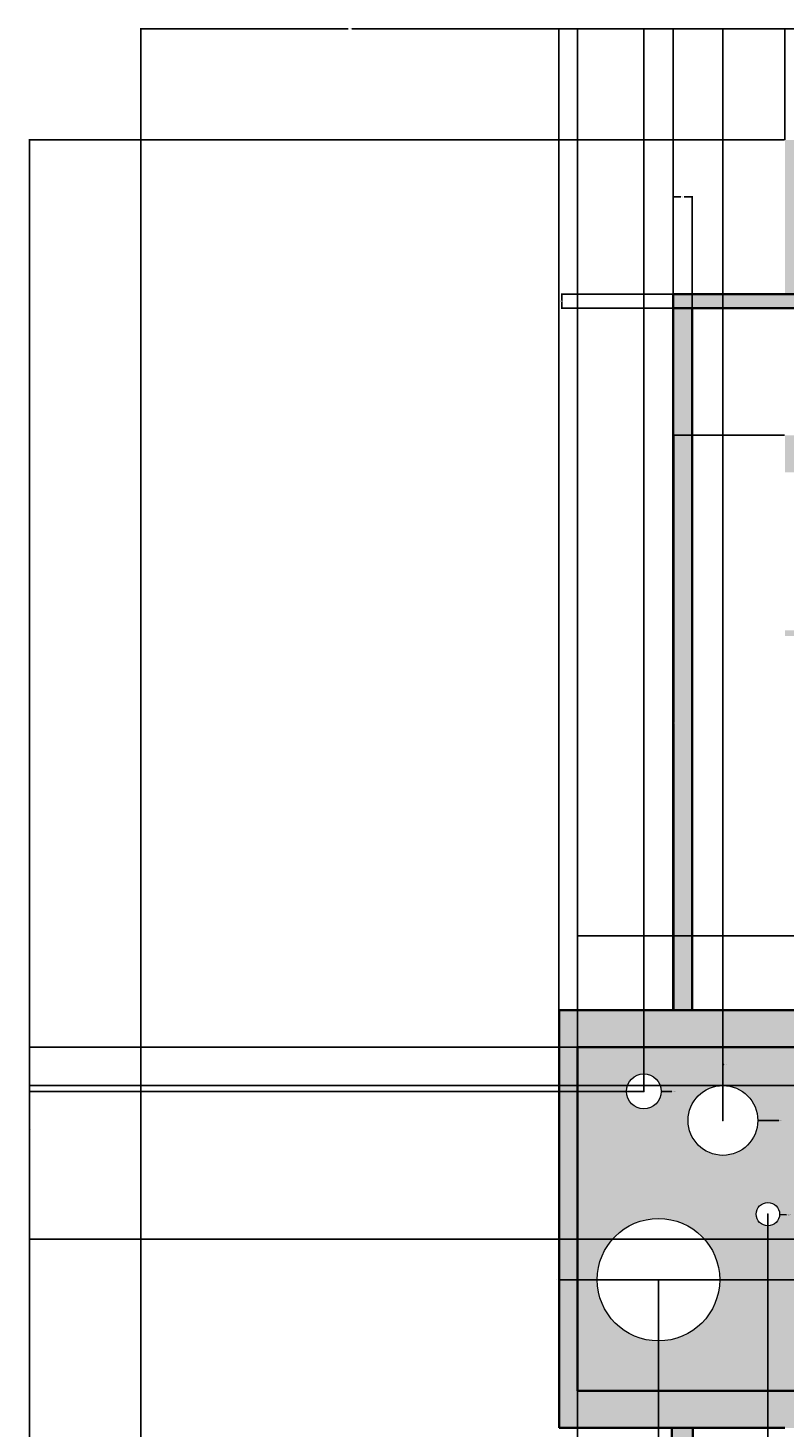
# Model space of a CAD drawing. Units: inches. Extents: x 73 to 607, y 92 to 651.
# Tile 13 of 18: x 73 to 256, y 311 to 651. Entities that reach past the tile are written whole.
import ezdxf

# ---------------------------------------------------------------- set-up
doc = ezdxf.new("R2010")
doc.units = ezdxf.units.IN
doc.header["$MEASUREMENT"] = 0
for name, color, linetype, lineweight in [('A-ANNO-DIMS', 2, 'Continuous', 18), ('A-ELEV', 7, 'Continuous', 35), ('A-ELEV-PANL', 7, 'Continuous', 18), ('A-ELEV-PATT-BKGD', 252, 'Continuous', 13), ('A-ELEV-PATT-SHAD', 8, 'Continuous', 13), ('A-ELEV-PATT-STON', 42, 'Continuous', 13), ('A-ELEV-PATT-WOOD', 32, 'Continuous', 13)]:
    doc.layers.add(name, color=color, linetype=linetype, lineweight=lineweight)
doc.styles.get("Standard").update_dxf_attribs({"font": 'arial.ttf'})
doc.dimstyles.get("Standard").update_dxf_attribs({"dimtxt": 0.18, "dimasz": 0.18, "dimexe": 0.18, "dimexo": 0.0625, "dimgap": 0.09, "dimtad": 0, "dimtih": 1, "dimtoh": 1, "dimdec": 4, "dimzin": 0, "dimdsep": 46, "dimtxsty": 'Standard', "dimcen": 0.09, "dimadec": 0, "dimazin": 0, "dimtfac": 1, "dimtdec": 4, "dimtofl": 0, "dimtmove": 0, "dimatfit": 3, "dimfxl": 1, "dimtolj": 1, "dimtzin": 0, "dimarcsym": 0})

# ---------------------------------------------------------------- blocks, each defined once
blk = doc.blocks.new('*D5')
at = {"layer": 'A-ANNO-DIMS', "color": 0, "lineweight": -2, "transparency": 16777216}
for p, q in [((256.41, 623.8), (72.92, 623.8)), ((73.1, 623.62), (73.1, 383.68)), ((73.1, 143.38), (73.1, 383.32)), ((100.04, 143.2), (72.92, 143.2))]:
    blk.add_line(p, q, dxfattribs=at)
at = {"layer": 'A-ANNO-DIMS', "color": 0, "transparency": 16777216}
for points in [[(73.07, 623.62), (73.13, 623.62), (73.1, 623.8)], [(73.07, 143.38), (73.13, 143.38), (73.1, 143.2)]]:
    blk.add_solid(points, dxfattribs=at)
at = {"layer": 'Defpoints', "color": 0, "transparency": 16777216}
for p in [(73.1, 623.8), (256.47, 623.8), (100.1, 143.2)]:
    blk.add_point(p, dxfattribs=at)
at = {"layer": 'A-ANNO-DIMS', "color": 0, "transparency": 16777216, "insert": (73.1, 383.5), "char_height": 0.18, "attachment_point": 5}
blk.add_mtext('\\A1;480.6', dxfattribs=at)
blk = doc.blocks.new('*D6')
at = {"layer": 'A-ANNO-DIMS', "color": 0, "lineweight": -2, "transparency": 16777216}
for p, q in [((100.1, 281.67), (100.1, 650.98)), ((100.28, 650.8), (150.41, 650.8)), ((201.45, 650.8), (151.32, 650.8)), ((201.63, 412.7), (201.63, 650.98))]:
    blk.add_line(p, q, dxfattribs=at)
at = {"layer": 'A-ANNO-DIMS', "color": 0, "transparency": 16777216}
for points in [[(100.28, 650.83), (100.28, 650.77), (100.1, 650.8)], [(201.45, 650.83), (201.45, 650.77), (201.63, 650.8)]]:
    blk.add_solid(points, dxfattribs=at)
at = {"layer": 'Defpoints', "color": 0, "transparency": 16777216}
for p in [(201.63, 650.8), (201.63, 412.64), (100.1, 281.6)]:
    blk.add_point(p, dxfattribs=at)
at = {"layer": 'A-ANNO-DIMS', "color": 0, "transparency": 16777216, "insert": (150.87, 650.8), "char_height": 0.18, "attachment_point": 5}
blk.add_mtext('\\A1;101.54', dxfattribs=at)
blk = doc.blocks.new('*D7')
at = {"layer": 'A-ANNO-DIMS', "color": 0, "lineweight": -2, "transparency": 16777216}
for p, q in [((201.63, 412.7), (201.63, 650.98)), ((201.81, 650.8), (215.01, 650.8)), ((229.14, 650.8), (215.94, 650.8)), ((229.32, 586.46), (229.32, 650.98))]:
    blk.add_line(p, q, dxfattribs=at)
at = {"layer": 'A-ANNO-DIMS', "color": 0, "transparency": 16777216}
for points in [[(201.81, 650.83), (201.81, 650.77), (201.63, 650.8)], [(229.14, 650.83), (229.14, 650.77), (229.32, 650.8)]]:
    blk.add_solid(points, dxfattribs=at)
at = {"layer": 'Defpoints', "color": 0, "transparency": 16777216}
for p in [(229.32, 650.8), (229.32, 586.39), (201.63, 412.64)]:
    blk.add_point(p, dxfattribs=at)
at = {"layer": 'A-ANNO-DIMS', "color": 0, "transparency": 16777216, "insert": (215.48, 650.8), "char_height": 0.18, "attachment_point": 5}
blk.add_mtext('\\A1;27.683', dxfattribs=at)
blk = doc.blocks.new('*D8')
at = {"layer": 'A-ANNO-DIMS', "color": 0, "lineweight": -2, "transparency": 16777216}
for p, q in [((229.32, 586.46), (229.32, 650.98)), ((229.5, 650.8), (242.43, 650.8)), ((256.29, 650.8), (243.36, 650.8)), ((256.47, 623.86), (256.47, 650.98))]:
    blk.add_line(p, q, dxfattribs=at)
at = {"layer": 'A-ANNO-DIMS', "color": 0, "transparency": 16777216}
for points in [[(229.5, 650.83), (229.5, 650.77), (229.32, 650.8)], [(256.29, 650.83), (256.29, 650.77), (256.47, 650.8)]]:
    blk.add_solid(points, dxfattribs=at)
at = {"layer": 'Defpoints', "color": 0, "transparency": 16777216}
for p in [(256.47, 650.8), (256.47, 623.8), (229.32, 586.39)]:
    blk.add_point(p, dxfattribs=at)
at = {"layer": 'A-ANNO-DIMS', "color": 0, "transparency": 16777216, "insert": (242.9, 650.8), "char_height": 0.18, "attachment_point": 5}
blk.add_mtext('\\A1;27.155', dxfattribs=at)
blk = doc.blocks.new('*D41')
at = {"layer": 'A-ANNO-DIMS', "color": 0, "lineweight": -2, "transparency": 16777216}
for p, q in [((229.26, 586.39), (202.14, 586.39)), ((202.32, 586.21), (202.32, 584.86)), ((202.32, 583.15), (202.32, 584.5)), ((229.26, 582.97), (202.14, 582.97))]:
    blk.add_line(p, q, dxfattribs=at)
at = {"layer": 'A-ANNO-DIMS', "color": 0, "transparency": 16777216}
for points in [[(202.29, 586.21), (202.35, 586.21), (202.32, 586.39)], [(202.29, 583.15), (202.35, 583.15), (202.32, 582.97)]]:
    blk.add_solid(points, dxfattribs=at)
at = {"layer": 'Defpoints', "color": 0, "transparency": 16777216}
for p in [(202.32, 586.39), (229.32, 586.39), (229.32, 582.97)]:
    blk.add_point(p, dxfattribs=at)
at = {"layer": 'A-ANNO-DIMS', "color": 0, "transparency": 16777216, "insert": (202.32, 584.68), "char_height": 0.18, "attachment_point": 5}
blk.add_mtext('\\A1;3.421', dxfattribs=at)
blk = doc.blocks.new('*D42')
at = {"layer": 'A-ANNO-DIMS', "color": 0, "lineweight": -2, "transparency": 16777216}
for p, q in [((229.32, 583.03), (229.32, 610.15)), ((229.5, 609.97), (231.22, 609.97)), ((233.74, 609.97), (232.02, 609.97)), ((233.92, 583.03), (233.92, 610.15))]:
    blk.add_line(p, q, dxfattribs=at)
at = {"layer": 'A-ANNO-DIMS', "color": 0, "transparency": 16777216}
for points in [[(229.5, 610), (229.5, 609.94), (229.32, 609.97)], [(233.74, 610), (233.74, 609.94), (233.92, 609.97)]]:
    blk.add_solid(points, dxfattribs=at)
at = {"layer": 'Defpoints', "color": 0, "transparency": 16777216}
for p in [(233.92, 609.97), (229.32, 582.97), (233.92, 582.97)]:
    blk.add_point(p, dxfattribs=at)
at = {"layer": 'A-ANNO-DIMS', "color": 0, "transparency": 16777216, "insert": (231.62, 609.97), "char_height": 0.18, "attachment_point": 5}
blk.add_mtext('\\A1;4.606', dxfattribs=at)
blk = doc.blocks.new('*D45')
at = {"layer": 'A-ANNO-DIMS', "color": 0, "lineweight": -2, "transparency": 16777216}
for p, q in [((256.41, 552.16), (229.29, 552.16)), ((229.47, 551.98), (229.47, 482.58)), ((229.47, 412.82), (229.47, 482.21)), ((256.41, 412.64), (229.29, 412.64))]:
    blk.add_line(p, q, dxfattribs=at)
at = {"layer": 'A-ANNO-DIMS', "color": 0, "transparency": 16777216}
for points in [[(229.44, 551.98), (229.5, 551.98), (229.47, 552.16)], [(229.44, 412.82), (229.5, 412.82), (229.47, 412.64)]]:
    blk.add_solid(points, dxfattribs=at)
at = {"layer": 'Defpoints', "color": 0, "transparency": 16777216}
for p in [(229.47, 552.16), (256.47, 552.16), (256.47, 412.64)]:
    blk.add_point(p, dxfattribs=at)
at = {"layer": 'A-ANNO-DIMS', "color": 0, "transparency": 16777216, "insert": (229.47, 482.4), "char_height": 0.18, "attachment_point": 5}
blk.add_mtext('\\A1;139.52', dxfattribs=at)
blk = doc.blocks.new('*D52')
at = {"layer": 'A-ANNO-DIMS', "color": 0, "lineweight": -2, "transparency": 16777216}
for p, q in [((206.13, 403.7), (206.13, 430.82)), ((206.31, 430.64), (323.93, 430.64)), ((442.34, 430.64), (324.72, 430.64)), ((442.52, 403.7), (442.52, 430.82))]:
    blk.add_line(p, q, dxfattribs=at)
at = {"layer": 'A-ANNO-DIMS', "color": 0, "transparency": 16777216}
for points in [[(206.31, 430.67), (206.31, 430.61), (206.13, 430.64)], [(442.34, 430.67), (442.34, 430.61), (442.52, 430.64)]]:
    blk.add_solid(points, dxfattribs=at)
at = {"layer": 'Defpoints', "color": 0, "transparency": 16777216}
for p in [(442.52, 430.64), (206.13, 403.64), (442.52, 403.64)]:
    blk.add_point(p, dxfattribs=at)
at = {"layer": 'A-ANNO-DIMS', "color": 0, "transparency": 16777216, "insert": (324.33, 430.64), "char_height": 0.18, "attachment_point": 5}
blk.add_mtext('\\A1;236.4', dxfattribs=at)
blk = doc.blocks.new('*D54')
at = {"layer": 'A-ANNO-DIMS', "color": 0, "lineweight": -2, "transparency": 16777216}
for p, q in [((206.13, 320.27), (206.13, 347.38)), ((206.31, 347.2), (275.84, 347.2)), ((346.14, 347.2), (276.61, 347.2)), ((346.32, 320.27), (346.32, 347.38))]:
    blk.add_line(p, q, dxfattribs=at)
at = {"layer": 'A-ANNO-DIMS', "color": 0, "transparency": 16777216}
for points in [[(206.31, 347.23), (206.31, 347.17), (206.13, 347.2)], [(346.14, 347.23), (346.14, 347.17), (346.32, 347.2)]]:
    blk.add_solid(points, dxfattribs=at)
at = {"layer": 'Defpoints', "color": 0, "transparency": 16777216}
for p in [(346.32, 347.2), (206.13, 320.2), (346.32, 320.2)]:
    blk.add_point(p, dxfattribs=at)
at = {"layer": 'A-ANNO-DIMS', "color": 0, "transparency": 16777216, "insert": (276.23, 347.2), "char_height": 0.18, "attachment_point": 5}
blk.add_mtext('\\A1;140.2', dxfattribs=at)
blk = doc.blocks.new('*D60')
at = {"layer": 'A-ANNO-DIMS', "color": 0, "lineweight": -2, "transparency": 16777216}
for p, q in [((225.69, 347.19), (225.87, 347.19)), ((225.78, 347.1), (225.78, 347.28)), ((249.57, 347.19), (240.83, 347.19))]:
    blk.add_line(p, q, dxfattribs=at)
at = {"layer": 'A-ANNO-DIMS', "color": 0, "transparency": 16777216}
blk.add_solid([(240.83, 347.22), (240.83, 347.16), (240.65, 347.19)], dxfattribs=at)
at = {"layer": 'Defpoints', "color": 0, "transparency": 16777216}
for p in [(210.91, 347.19), (240.65, 347.19)]:
    blk.add_point(p, dxfattribs=at)
at = {"layer": 'A-ANNO-DIMS', "color": 0, "transparency": 16777216, "insert": (250.06, 347.19), "char_height": 0.18, "attachment_point": 5}
blk.add_mtext('\\A1;∅29.74', dxfattribs=at)
blk = doc.blocks.new('*D63')
at = {"layer": 'A-ANNO-DIMS', "color": 0, "lineweight": -2, "transparency": 16777216}
for p, q in [((241.34, 385.85), (241.52, 385.85)), ((241.43, 385.76), (241.43, 385.94)), ((254.98, 385.85), (250.07, 385.85))]:
    blk.add_line(p, q, dxfattribs=at)
at = {"layer": 'A-ANNO-DIMS', "color": 0, "transparency": 16777216}
blk.add_solid([(250.07, 385.88), (250.07, 385.82), (249.89, 385.85)], dxfattribs=at)
at = {"layer": 'Defpoints', "color": 0, "transparency": 16777216}
for p in [(232.96, 385.85), (249.89, 385.85)]:
    blk.add_point(p, dxfattribs=at)
at = {"layer": 'A-ANNO-DIMS', "color": 0, "transparency": 16777216, "insert": (255.54, 385.85), "char_height": 0.18, "attachment_point": 5}
blk.add_mtext('\\A1;∅16.935', dxfattribs=at)
blk = doc.blocks.new('*D68')
at = {"layer": 'A-ANNO-DIMS', "color": 0, "lineweight": -2, "transparency": 16777216}
for p, q in [((206.13, 403.7), (206.13, 650.98)), ((206.31, 650.8), (213.72, 650.8)), ((222.04, 650.8), (214.63, 650.8)), ((222.22, 392.97), (222.22, 650.98))]:
    blk.add_line(p, q, dxfattribs=at)
at = {"layer": 'A-ANNO-DIMS', "color": 0, "transparency": 16777216}
for points in [[(206.31, 650.83), (206.31, 650.77), (206.13, 650.8)], [(222.04, 650.83), (222.04, 650.77), (222.22, 650.8)]]:
    blk.add_solid(points, dxfattribs=at)
at = {"layer": 'Defpoints', "color": 0, "transparency": 16777216}
for p in [(222.22, 650.8), (206.13, 403.64), (222.22, 392.9)]:
    blk.add_point(p, dxfattribs=at)
at = {"layer": 'A-ANNO-DIMS', "color": 0, "transparency": 16777216, "insert": (214.18, 650.8), "char_height": 0.18, "attachment_point": 5}
blk.add_mtext('\\A1;16.085', dxfattribs=at)
blk = doc.blocks.new('*D69')
at = {"layer": 'A-ANNO-DIMS', "color": 0, "lineweight": -2, "transparency": 16777216}
for p, q in [((222.22, 392.97), (222.22, 650.98)), ((222.4, 650.8), (231.46, 650.8)), ((241.25, 650.8), (232.19, 650.8)), ((241.43, 385.91), (241.43, 650.98))]:
    blk.add_line(p, q, dxfattribs=at)
at = {"layer": 'A-ANNO-DIMS', "color": 0, "transparency": 16777216}
for points in [[(222.4, 650.83), (222.4, 650.77), (222.22, 650.8)], [(241.25, 650.83), (241.25, 650.77), (241.43, 650.8)]]:
    blk.add_solid(points, dxfattribs=at)
at = {"layer": 'Defpoints', "color": 0, "transparency": 16777216}
for p in [(241.43, 650.8), (222.22, 392.9), (241.43, 385.85)]:
    blk.add_point(p, dxfattribs=at)
at = {"layer": 'A-ANNO-DIMS', "color": 0, "transparency": 16777216, "insert": (231.82, 650.8), "char_height": 0.18, "attachment_point": 5}
blk.add_mtext('\\A1;19.21', dxfattribs=at)
blk = doc.blocks.new('*D70')
at = {"layer": 'A-ANNO-DIMS', "color": 0, "lineweight": -2, "transparency": 16777216}
for p, q in [((241.43, 385.91), (241.43, 650.98)), ((241.61, 650.8), (252.54, 650.8)), ((264.41, 650.8), (253.47, 650.8)), ((264.59, 394.38), (264.59, 650.98))]:
    blk.add_line(p, q, dxfattribs=at)
at = {"layer": 'A-ANNO-DIMS', "color": 0, "transparency": 16777216}
for points in [[(241.61, 650.83), (241.61, 650.77), (241.43, 650.8)], [(264.41, 650.83), (264.41, 650.77), (264.59, 650.8)]]:
    blk.add_solid(points, dxfattribs=at)
at = {"layer": 'Defpoints', "color": 0, "transparency": 16777216}
for p in [(264.59, 650.8), (264.59, 394.31), (241.43, 385.85)]:
    blk.add_point(p, dxfattribs=at)
at = {"layer": 'A-ANNO-DIMS', "color": 0, "transparency": 16777216, "insert": (253.01, 650.8), "char_height": 0.18, "attachment_point": 5}
blk.add_mtext('\\A1;23.163', dxfattribs=at)
blk = doc.blocks.new('*D73')
at = {"layer": 'A-ANNO-DIMS', "color": 0, "lineweight": -2, "transparency": 16777216}
for p, q in [((225.78, 347.13), (225.78, 116.02)), ((206.13, 320.14), (206.13, 116.02)), ((206.31, 116.2), (215.5, 116.2)), ((225.6, 116.2), (216.41, 116.2))]:
    blk.add_line(p, q, dxfattribs=at)
at = {"layer": 'A-ANNO-DIMS', "color": 0, "transparency": 16777216}
for points in [[(206.31, 116.23), (206.31, 116.17), (206.13, 116.2)], [(225.6, 116.23), (225.6, 116.17), (225.78, 116.2)]]:
    blk.add_solid(points, dxfattribs=at)
at = {"layer": 'Defpoints', "color": 0, "transparency": 16777216}
for p in [(225.78, 347.19), (206.13, 320.2), (225.78, 116.2)]:
    blk.add_point(p, dxfattribs=at)
at = {"layer": 'A-ANNO-DIMS', "color": 0, "transparency": 16777216, "insert": (215.96, 116.2), "char_height": 0.18, "attachment_point": 5}
blk.add_mtext('\\A1;19.645', dxfattribs=at)
blk = doc.blocks.new('*D74')
at = {"layer": 'A-ANNO-DIMS', "color": 0, "lineweight": -2, "transparency": 16777216}
for p, q in [((252.34, 363.04), (252.34, 116.02)), ((225.78, 347.13), (225.78, 116.02)), ((225.96, 116.2), (238.66, 116.2)), ((252.16, 116.2), (239.46, 116.2))]:
    blk.add_line(p, q, dxfattribs=at)
at = {"layer": 'A-ANNO-DIMS', "color": 0, "transparency": 16777216}
for points in [[(225.96, 116.23), (225.96, 116.17), (225.78, 116.2)], [(252.16, 116.23), (252.16, 116.17), (252.34, 116.2)]]:
    blk.add_solid(points, dxfattribs=at)
at = {"layer": 'Defpoints', "color": 0, "transparency": 16777216}
for p in [(252.34, 363.11), (225.78, 347.19), (252.34, 116.2)]:
    blk.add_point(p, dxfattribs=at)
at = {"layer": 'A-ANNO-DIMS', "color": 0, "transparency": 16777216, "insert": (239.06, 116.2), "char_height": 0.18, "attachment_point": 5}
blk.add_mtext('\\A1;26.56', dxfattribs=at)
blk = doc.blocks.new('*D75')
at = {"layer": 'A-ANNO-DIMS', "color": 0, "lineweight": -2, "transparency": 16777216}
for p, q in [((252.34, 363.04), (252.34, 116.02)), ((267.42, 345.14), (267.42, 116.02)), ((252.52, 116.2), (259.42, 116.2)), ((267.24, 116.2), (260.33, 116.2))]:
    blk.add_line(p, q, dxfattribs=at)
at = {"layer": 'A-ANNO-DIMS', "color": 0, "transparency": 16777216}
for points in [[(252.52, 116.23), (252.52, 116.17), (252.34, 116.2)], [(267.24, 116.23), (267.24, 116.17), (267.42, 116.2)]]:
    blk.add_solid(points, dxfattribs=at)
at = {"layer": 'Defpoints', "color": 0, "transparency": 16777216}
for p in [(252.34, 363.11), (267.42, 345.2), (267.42, 116.2)]:
    blk.add_point(p, dxfattribs=at)
at = {"layer": 'A-ANNO-DIMS', "color": 0, "transparency": 16777216, "insert": (259.88, 116.2), "char_height": 0.18, "attachment_point": 5}
blk.add_mtext('\\A1;15.074', dxfattribs=at)
blk = doc.blocks.new('*D78')
at = {"layer": 'A-ANNO-DIMS', "color": 0, "lineweight": -2, "transparency": 16777216}
for p, q in [((206.07, 403.64), (72.92, 403.64)), ((73.1, 403.46), (73.1, 398.45)), ((73.1, 393.08), (73.1, 398.09)), ((222.16, 392.9), (72.92, 392.9))]:
    blk.add_line(p, q, dxfattribs=at)
at = {"layer": 'A-ANNO-DIMS', "color": 0, "transparency": 16777216}
for points in [[(73.07, 403.46), (73.13, 403.46), (73.1, 403.64)], [(73.07, 393.08), (73.13, 393.08), (73.1, 392.9)]]:
    blk.add_solid(points, dxfattribs=at)
at = {"layer": 'Defpoints', "color": 0, "transparency": 16777216}
for p in [(206.13, 403.64), (73.1, 392.9), (222.22, 392.9)]:
    blk.add_point(p, dxfattribs=at)
at = {"layer": 'A-ANNO-DIMS', "color": 0, "transparency": 16777216, "insert": (73.1, 398.27), "char_height": 0.18, "attachment_point": 5}
blk.add_mtext('\\A1;10.733', dxfattribs=at)
blk = doc.blocks.new('*D80')
at = {"layer": 'A-ANNO-DIMS', "color": 0, "lineweight": -2, "transparency": 16777216}
for p, q in [((316.22, 394.31), (72.92, 394.31)), ((73.1, 394.13), (73.1, 375.87)), ((73.1, 357.24), (73.1, 375.5)), ((321.31, 357.06), (72.92, 357.06))]:
    blk.add_line(p, q, dxfattribs=at)
at = {"layer": 'A-ANNO-DIMS', "color": 0, "transparency": 16777216}
for points in [[(73.07, 394.13), (73.13, 394.13), (73.1, 394.31)], [(73.07, 357.24), (73.13, 357.24), (73.1, 357.06)]]:
    blk.add_solid(points, dxfattribs=at)
at = {"layer": 'Defpoints', "color": 0, "transparency": 16777216}
for p in [(316.28, 394.31), (73.1, 357.06), (321.37, 357.06)]:
    blk.add_point(p, dxfattribs=at)
at = {"layer": 'A-ANNO-DIMS', "color": 0, "transparency": 16777216, "insert": (73.1, 375.69), "char_height": 0.18, "attachment_point": 5}
blk.add_mtext('\\A1;37.26', dxfattribs=at)
blk = doc.blocks.new('*D132')
at = {"layer": 'A-ANNO-DIMS', "color": 0, "lineweight": -2, "transparency": 16777216}
for p, q in [((222.13, 392.9), (222.31, 392.9)), ((222.22, 392.81), (222.22, 392.99)), ((229, 392.9), (226.64, 392.9))]:
    blk.add_line(p, q, dxfattribs=at)
at = {"layer": 'A-ANNO-DIMS', "color": 0, "transparency": 16777216}
blk.add_solid([(226.64, 392.93), (226.64, 392.87), (226.46, 392.9)], dxfattribs=at)
at = {"layer": 'Defpoints', "color": 0, "transparency": 16777216}
for p in [(217.98, 392.91), (226.46, 392.9)]:
    blk.add_point(p, dxfattribs=at)
at = {"layer": 'A-ANNO-DIMS', "color": 0, "transparency": 16777216, "insert": (229.49, 392.9), "char_height": 0.18, "attachment_point": 5}
blk.add_mtext('\\A1;∅8.474', dxfattribs=at)
blk = doc.blocks.new('*D133')
at = {"layer": 'A-ANNO-DIMS', "color": 0, "lineweight": -2, "transparency": 16777216}
for p, q in [((241.61, 399.39), (241.43, 399.39)), ((241.43, 399.39), (241.43, 394.49)), ((241.34, 385.85), (241.52, 385.85)), ((241.43, 385.76), (241.43, 385.94))]:
    blk.add_line(p, q, dxfattribs=at)
at = {"layer": 'A-ANNO-DIMS', "color": 0, "transparency": 16777216}
blk.add_solid([(241.4, 394.49), (241.46, 394.49), (241.43, 394.31)], dxfattribs=at)
at = {"layer": 'Defpoints', "color": 0, "transparency": 16777216}
for p in [(241.43, 394.31), (241.42, 377.38)]:
    blk.add_point(p, dxfattribs=at)
at = {"layer": 'A-ANNO-DIMS', "color": 0, "transparency": 16777216, "insert": (242.17, 399.39), "char_height": 0.18, "attachment_point": 5}
blk.add_mtext('\\A1;∅16.935', dxfattribs=at)
blk = doc.blocks.new('*D137')
at = {"layer": 'A-ANNO-DIMS', "color": 0, "lineweight": -2, "transparency": 16777216}
for p, q in [((252.25, 363.11), (252.43, 363.11)), ((252.34, 363.02), (252.34, 363.2)), ((256.88, 362.94), (255.36, 363))]:
    blk.add_line(p, q, dxfattribs=at)
at = {"layer": 'A-ANNO-DIMS', "color": 0, "transparency": 16777216}
blk.add_solid([(255.36, 363.03), (255.36, 362.97), (255.18, 363)], dxfattribs=at)
at = {"layer": 'Defpoints', "color": 0, "transparency": 16777216}
for p in [(249.5, 363.21), (255.18, 363)]:
    blk.add_point(p, dxfattribs=at)
at = {"layer": 'A-ANNO-DIMS', "color": 0, "transparency": 16777216, "insert": (257.37, 362.94), "char_height": 0.18, "attachment_point": 5}
blk.add_mtext('\\A1;∅5.679', dxfattribs=at)
blk = doc.blocks.new('*D139')
at = {"layer": 'A-ANNO-DIMS', "color": 0, "lineweight": -2, "transparency": 16777216}
for p, q in [((201.99, 347.19), (210.73, 347.19)), ((225.69, 347.19), (225.87, 347.19)), ((225.78, 347.1), (225.78, 347.28))]:
    blk.add_line(p, q, dxfattribs=at)
at = {"layer": 'A-ANNO-DIMS', "color": 0, "transparency": 16777216}
blk.add_solid([(210.73, 347.22), (210.73, 347.16), (210.91, 347.19)], dxfattribs=at)
at = {"layer": 'Defpoints', "color": 0, "transparency": 16777216}
for p in [(210.91, 347.19), (240.65, 347.2)]:
    blk.add_point(p, dxfattribs=at)
at = {"layer": 'A-ANNO-DIMS', "color": 0, "transparency": 16777216, "insert": (201.49, 347.19), "char_height": 0.18, "attachment_point": 5}
blk.add_mtext('\\A1;∅29.74', dxfattribs=at)

msp = doc.modelspace()

# ---------------------------------------------------------------- hatches: boundary and pattern name
at = {"layer": 'A-ELEV-PATT-BKGD'}
h = msp.add_hatch(color=256, dxfattribs=at)
h.dxf.hatch_style = 1
h.paths.add_polyline_path([(321.3008, 479.2042), (312.3008, 479.2042), (312.3008, 478.7576), (312.3008, 412.636), (321.3008, 412.636)])
h.paths.add_polyline_path([(312.3008, 504.7576), (256.4726, 504.7576), (256.4726, 503.4576), (312.3008, 503.4576)], flags=17)
h.paths.add_polyline_path([(321.3008, 543.1576), (321.3008, 552.1576), (320.3257, 552.1576), (312.3008, 552.1576), (256.4726, 552.1576), (256.4726, 543.1576), (312.3008, 543.1576), (312.3008, 479.2042), (321.3008, 479.2042)])
h.paths.add_polyline_path([(451.5214, 412.636), (256.4726, 412.636), (256.4726, 403.636), (442.5214, 403.636), (442.5214, 320.2042), (206.1343, 320.2042), (206.1343, 320.9135), (206.1343, 403.636), (256.4726, 403.636), (256.4726, 412.636), (201.6343, 412.636), (201.6343, 320.9135), (201.6343, 320.2042), (201.6343, 311.2042), (256.4726, 311.2042), (451.5214, 311.2042)])
h.paths.add_polyline_path([(431.07, 258.6914), (369.5339, 258.6914), (369.5339, 247.4054), (396.692, 247.4054), (425.07, 247.4054), (425.07, 194.7312), (396.692, 194.6197), (396.692, 194.5366), (369.5339, 194.5366), (369.5339, 185.6619), (431.07, 185.6619)])
h.paths.add_polyline_path([(580.0983, 262.3024), (451.5214, 262.3024), (451.5214, 143.2042), (580.0983, 143.2042)])
h.paths.add_polyline_path([(454.7049, 174.802), (454.7049, 256.6321), (577.9249, 256.6321), (577.9249, 174.802)], flags=16)
h.paths.add_polyline_path([(465.9716, 191.1416, -1), (473.7874, 191.1416, -1)], flags=0)
h.paths.add_polyline_path([(490.5373, 181.6586, -1), (494.9999, 181.6586, -1)], flags=0)
h.paths.add_polyline_path([(476.2996, 209.8287, -1), (500.5844, 209.8287, -1)], flags=0)
h.paths.add_polyline_path([(505.3326, 194.7675, -1), (512.5843, 194.7675, -1)], flags=0)
h.paths.add_polyline_path([(520.9613, 186.679, -1), (526.544, 186.679, -1)], flags=0)
h.paths.add_polyline_path([(466.8103, 225.7267, -1), (470.1573, 225.7267, -1)], flags=0)
h.paths.add_polyline_path([(527.1059, 203.6926, -1), (536.0311, 203.6926, -1)], flags=0)
h.paths.add_polyline_path([(504.775, 232.6995, -1), (513.7002, 232.6995, -1)], flags=0)
h.paths.add_polyline_path([(546.9241, 183.611, -1), (554.7336, 183.611, -1)], flags=0)
h.paths.add_polyline_path([(459.5544, 243.856, -1), (466.8061, 243.856, -1)], flags=0)
h.paths.add_polyline_path([(476.3045, 246.924, -1), (488.5767, 246.924, -1)], flags=0)
h.paths.add_polyline_path([(529.9044, 226.8424, -1), (556.68, 226.8424, -1)], flags=0)
h.paths.add_polyline_path([(554.1814, 203.9716, -1), (561.4331, 203.9716, -1)], flags=0)
h.paths.add_polyline_path([(567.8561, 193.3729, -1), (570.6475, 193.3729, -1)], flags=0)
h.paths.add_polyline_path([(522.3584, 250.271, -1), (525.7053, 250.271, -1)], flags=0)
h.paths.add_polyline_path([(561.9965, 245.2506, -1), (567.5748, 245.2506, -1)], flags=0)
h.paths.add_polyline_path([(347.8686, 194.5366), (341.8686, 194.5366), (341.8686, 194.5452), (314.0144, 194.5452), (314.0144, 188.5452), (347.8686, 188.5452)])
h.paths.add_polyline_path([(347.8686, 253.4054), (314.0144, 253.4054), (314.0144, 247.4054), (341.8686, 247.4054), (347.8686, 247.4054)])
h.paths.add_polyline_path([(304.3559, 253.4054), (298.3559, 253.4054), (298.3559, 188.5452), (304.3559, 188.5452)])
h.paths.add_polyline_path([(450.6603, 552.1576), (369.9727, 552.1576), (369.9727, 479.2042), (374.4727, 479.2042), (374.4727, 547.6576), (446.1603, 547.6576), (446.1603, 479.2042), (450.6603, 479.2042)])
h.paths.add_polyline_path([(374.4727, 479.2042), (369.9727, 479.2042), (369.9727, 465.0632), (374.4727, 465.0632)])
h.paths.add_polyline_path([(450.6603, 479.2042), (446.1603, 479.2042), (446.1603, 465.0632), (450.6603, 465.0632)])
h.paths.add_polyline_path([(256.4726, 281.6039), (109.0983, 281.6039), (100.0983, 281.6039), (100.0983, 167.2042), (100.0983, 143.2042), (109.0983, 143.2042), (109.0983, 167.2042), (109.0983, 272.6039), (256.4726, 272.6039)])
at = {"layer": 'A-ELEV-PATT-SHAD'}
h = msp.add_hatch(color=256, dxfattribs=at)
h.dxf.hatch_style = 1
h.paths.add_polyline_path([(451.5214, 412.636), (256.4726, 412.636), (256.4726, 403.636), (442.5214, 403.636), (442.5214, 320.2042), (206.1343, 320.2042), (206.1343, 320.9135), (206.1343, 403.636), (256.4726, 403.636), (256.4726, 412.636), (201.6343, 412.636), (201.6343, 320.9135), (201.6343, 320.2042), (201.6343, 311.2042), (256.4726, 311.2042), (451.5214, 311.2042)])
h.paths.add_polyline_path([(580.0983, 262.3024), (451.5214, 262.3024), (451.5214, 143.2042), (580.0983, 143.2042)])
h.paths.add_polyline_path([(454.7049, 174.802), (454.7049, 256.6321), (577.9249, 256.6321), (577.9249, 174.802)], flags=16)
h.paths.add_polyline_path([(465.9716, 191.1416, -1), (473.7874, 191.1416, -1)], flags=0)
h.paths.add_polyline_path([(490.5373, 181.6586, -1), (494.9999, 181.6586, -1)], flags=0)
h.paths.add_polyline_path([(476.2996, 209.8287, -1), (500.5844, 209.8287, -1)], flags=0)
h.paths.add_polyline_path([(505.3326, 194.7675, -1), (512.5843, 194.7675, -1)], flags=0)
h.paths.add_polyline_path([(520.9613, 186.679, -1), (526.544, 186.679, -1)], flags=0)
h.paths.add_polyline_path([(466.8103, 225.7267, -1), (470.1573, 225.7267, -1)], flags=0)
h.paths.add_polyline_path([(527.1059, 203.6926, -1), (536.0311, 203.6926, -1)], flags=0)
h.paths.add_polyline_path([(459.5544, 243.856, -1), (466.8061, 243.856, -1)], flags=0)
h.paths.add_polyline_path([(504.775, 232.6995, -1), (513.7002, 232.6995, -1)], flags=0)
h.paths.add_polyline_path([(476.3045, 246.924, -1), (488.5767, 246.924, -1)], flags=0)
h.paths.add_polyline_path([(546.9241, 183.611, -1), (554.7336, 183.611, -1)], flags=0)
h.paths.add_polyline_path([(529.9044, 226.8424, -1), (556.68, 226.8424, -1)], flags=0)
h.paths.add_polyline_path([(554.1814, 203.9716, -1), (561.4331, 203.9716, -1)], flags=0)
h.paths.add_polyline_path([(522.3584, 250.271, -1), (525.7053, 250.271, -1)], flags=0)
h.paths.add_polyline_path([(567.8561, 193.3729, -1), (570.6475, 193.3729, -1)], flags=0)
h.paths.add_polyline_path([(561.9965, 245.2506, -1), (567.5748, 245.2506, -1)], flags=0)
h.paths.add_polyline_path([(431.07, 258.6914), (369.5339, 258.6914), (369.5339, 247.4054), (396.692, 247.4054), (425.07, 247.4054), (425.07, 194.7312), (396.692, 194.6197), (396.692, 194.5366), (369.5339, 194.5366), (369.5339, 185.6619), (431.07, 185.6619)])
h.paths.add_polyline_path([(347.8686, 253.4054), (314.0144, 253.4054), (314.0144, 247.4054), (341.8686, 247.4054), (347.8686, 247.4054)])
h.paths.add_polyline_path([(304.3559, 253.4054), (298.3559, 253.4054), (298.3559, 188.5452), (304.3559, 188.5452)])
h.paths.add_polyline_path([(347.8686, 194.5366), (341.8686, 194.5366), (341.8686, 194.5452), (314.0144, 194.5452), (314.0144, 188.5452), (347.8686, 188.5452)])
at = {"layer": 'A-ELEV-PATT-STON'}
h = msp.add_hatch(color=256, dxfattribs=at)
h.dxf.hatch_style = 1
h.paths.add_polyline_path([(394.7799, 623.801), (256.4726, 623.801), (256.4726, 586.3933), (394.7799, 586.3933)])
h.paths.add_polyline_path([(233.924, 582.9721), (229.3177, 582.9721), (229.3177, 412.636), (233.924, 412.636)])
h.paths.add_polyline_path([(234.1465, 311.2042), (229.0534, 311.2042), (229.0534, 281.6039), (234.1465, 281.6039)])
h.paths.add_polyline_path([(234.384, 272.6039), (228.8076, 272.6039), (228.8076, 167.2042), (234.384, 167.2042)])
at = {"layer": 'A-ELEV-PATT-WOOD'}
h = msp.add_hatch(color=256, dxfattribs=at)
h.dxf.hatch_style = 1
h.paths.add_polyline_path([(394.7799, 586.3933), (229.3177, 586.3933), (229.3177, 582.9721), (394.7799, 582.9721)])
h = msp.add_hatch(color=256, dxfattribs=at)
h.dxf.hatch_style = 1
h.paths.add_polyline_path([(256.4726, 403.636), (206.1343, 403.636), (206.1343, 320.9135), (206.1343, 320.2042), (256.4726, 320.2042)])
h.paths.add_polyline_path([(217.9817, 392.9028, -1), (226.456, 392.9028, -1)], flags=16)
h.paths.add_polyline_path([(232.9598, 385.8466, -1), (249.8948, 385.8466, -1)], flags=16)
h.paths.add_polyline_path([(240.6496, 347.1939, -1), (210.9085, 347.1939, -1)], flags=16)
h.paths.add_polyline_path([(255.1802, 363.1072, -1), (249.5015, 363.1072, -1)], flags=16)
h.paths.add_polyline_path([(334.6695, 403.636), (256.4726, 403.636), (256.4726, 320.2042), (334.6695, 320.2042)])
h.paths.add_polyline_path([(312.5994, 370.2541, -1), (276.6709, 370.2541, -1)], flags=16)
h.paths.add_polyline_path([(260.9211, 394.3141, -1), (268.2596, 394.3141, -1)], flags=16)
h.paths.add_polyline_path([(273.3424, 345.2025, -1), (261.4879, 345.2025, -1)], flags=16)
h.paths.add_polyline_path([(302.1597, 335.0415, -1), (291.9906, 335.0415, -1)], flags=16)
h.paths.add_polyline_path([(312.0498, 394.3141, -1), (320.5173, 394.3141, -1)], flags=16)
h.paths.add_polyline_path([(325.3197, 357.0571, -1), (317.4166, 357.0571, -1)], flags=16)

# ---------------------------------------------------------------- linework, layer by layer
at = {"layer": 'A-ELEV'}
for p, q in [((451.5214, 412.636), (201.6343, 412.636)), ((201.6343, 412.636), (201.6343, 320.9135)), ((442.5214, 403.636), (206.1343, 403.636)), ((206.1343, 403.636), (206.1343, 320.9135)), ((201.6343, 320.9135), (201.6343, 320.2042)), ((201.6343, 311.2042), (201.6343, 320.2042)), ((206.1343, 320.9135), (206.1343, 320.2042)), ((206.1343, 320.2042), (442.5214, 320.2042)), ((256.4726, 311.2042), (201.6343, 311.2042))]:
    msp.add_line(p, q, dxfattribs=at)
for points in [[(229.3177, 582.9721), (394.7799, 582.9721), (394.7799, 586.3933), (229.3177, 586.3933)], [(229.3177, 412.636), (233.924, 412.636), (233.924, 582.9721), (229.3177, 582.9721)], [(229.0534, 311.2042), (234.1465, 311.2042), (234.1465, 281.6039), (229.0534, 281.6039)]]:
    msp.add_lwpolyline(points, close=True, dxfattribs=at)
at = {"layer": 'A-ELEV-PANL'}
for centre, radius in [((222.2189, 392.9028), 4.2371), ((241.4273, 385.8466), 8.4675), ((252.3408, 363.1072), 2.8393), ((225.7791, 347.1939), 14.8705)]:
    msp.add_circle(centre, radius, dxfattribs=at)

# ---------------------------------------------------------------- dimensions: what is measured, and where the dimension line sits
at = {"layer": 'A-ANNO-DIMS'}
for base, p1, p2, override, picture, middle in [((201.6343, 650.801), (100.0983, 281.6039), (201.6343, 412.636), {"dimdec": 2, "dimlfac": 1, "dimrnd": 0, "dimzin": 0, "dimdsep": 46, "dimlunit": 2}, '*D6', (150.8663, 650.801)), ((229.3177, 650.801), (201.6343, 412.636), (229.3177, 586.3933), {"dimdec": 3, "dimlfac": 1, "dimrnd": 0, "dimzin": 0, "dimdsep": 46, "dimlunit": 2}, '*D7', (215.476, 650.801)), ((222.2189, 650.801), (206.1343, 403.636), (222.2189, 392.9028), {"dimdec": 3, "dimlfac": 1, "dimrnd": 0, "dimzin": 0, "dimdsep": 46, "dimlunit": 2}, '*D68', (214.1766, 650.801)), ((241.4273, 650.801), (222.2189, 392.9028), (241.4273, 385.8466), {"dimdec": 2, "dimlfac": 1, "dimrnd": 0, "dimzin": 0, "dimdsep": 46, "dimlunit": 2}, '*D69', (231.8231, 650.801)), ((256.4726, 650.801), (229.3177, 586.3933), (256.4726, 623.801), {"dimdec": 3, "dimlfac": 1, "dimrnd": 0, "dimzin": 0, "dimdsep": 46, "dimlunit": 2}, '*D8', (242.8951, 650.801)), ((264.5904, 650.801), (241.4273, 385.8466), (264.5904, 394.3141), {"dimdec": 3, "dimlfac": 1, "dimrnd": 0, "dimzin": 0, "dimdsep": 46, "dimlunit": 2}, '*D70', (253.0088, 650.801)), ((233.924, 609.9721), (229.3177, 582.9721), (233.924, 582.9721), {"dimdec": 3, "dimlfac": 1, "dimrnd": 0, "dimzin": 0, "dimdsep": 46, "dimlunit": 2}, '*D42', (231.6209, 609.9721)), ((442.5214, 430.636), (206.1343, 403.636), (442.5214, 403.636), {"dimdec": 1, "dimlfac": 1, "dimrnd": 0, "dimzin": 0, "dimdsep": 46, "dimlunit": 2}, '*D52', (324.3278, 430.636)), ((252.3408, 116.2042), (225.7791, 347.1939), (252.3408, 363.1072), {"dimdec": 2, "dimlfac": 1, "dimrnd": 0, "dimzin": 0, "dimdsep": 46, "dimlunit": 2}, '*D74', (239.0599, 116.2042)), ((267.4151, 116.2042), (252.3408, 363.1072), (267.4151, 345.2025), {"dimdec": 3, "dimlfac": 1, "dimrnd": 0, "dimzin": 0, "dimdsep": 46, "dimlunit": 2}, '*D75', (259.878, 116.2042)), ((346.3213, 347.2042), (206.1343, 320.2042), (346.3213, 320.2042), {"dimdec": 1, "dimlfac": 1, "dimrnd": 0, "dimzin": 0, "dimdsep": 46, "dimlunit": 2}, '*D54', (276.2278, 347.2042)), ((225.7791, 116.2042), (206.1343, 320.2042), (225.7791, 347.1939), {"dimdec": 3, "dimlfac": 1, "dimrnd": 0, "dimzin": 0, "dimdsep": 46, "dimlunit": 2}, '*D73', (215.9567, 116.2042))]:
    dim = msp.add_linear_dim(base=base, p1=p1, p2=p2, dimstyle='Standard', override=override, dxfattribs=at)
    dim.commit()
    dim.dimension.update_dxf_attribs({"geometry": picture, "text_midpoint": middle})
for base, p1, p2, override, picture, middle in [((73.0983, 623.801), (100.0983, 143.2042), (256.4726, 623.801), {"dimdec": 1, "dimlfac": 1, "dimrnd": 0, "dimzin": 0, "dimdsep": 46, "dimlunit": 2}, '*D5', (73.0983, 383.5026)), ((202.3177, 586.3933), (229.3177, 582.9721), (229.3177, 586.3933), {"dimdec": 3, "dimlfac": 1, "dimrnd": 0, "dimzin": 0, "dimdsep": 46, "dimlunit": 2}, '*D41', (202.3177, 584.6827)), ((229.4726, 552.1576), (256.4726, 412.636), (256.4726, 552.1576), {"dimdec": 2, "dimlfac": 1, "dimrnd": 0, "dimzin": 0, "dimdsep": 46, "dimlunit": 2}, '*D45', (229.4726, 482.3968)), ((73.0983, 392.9028), (206.1343, 403.636), (222.2189, 392.9028), {"dimdec": 3, "dimlfac": 1, "dimrnd": 0, "dimzin": 0, "dimdsep": 46, "dimlunit": 2}, '*D78', (73.0983, 398.2694)), ((73.0983, 357.0571), (316.2836, 394.3141), (321.3681, 357.0571), {"dimdec": 2, "dimlfac": 1, "dimrnd": 0, "dimzin": 0, "dimdsep": 46, "dimlunit": 2}, '*D80', (73.0983, 375.6856))]:
    dim = msp.add_linear_dim(base=base, p1=p1, p2=p2, angle=90, dimstyle='Standard', override=override, dxfattribs=at)
    dim.commit()
    dim.dimension.update_dxf_attribs({"geometry": picture, "text_midpoint": middle})
for p1, p2, override, picture, middle in [((241.4245, 377.3791), (241.43, 394.3141), {"dimdec": 3, "dimlfac": 1, "dimrnd": 0, "dimzin": 0, "dimdsep": 46, "dimlunit": 2}, '*D133', (242.1739, 399.3946)), ((217.9817, 392.9057), (226.456, 392.9), {"dimdec": 3, "dimlfac": 1, "dimrnd": 0, "dimzin": 0, "dimdsep": 46, "dimlunit": 2}, '*D132', (228.9983, 392.8983)), ((232.9598, 385.8462), (249.8948, 385.847), {"dimdec": 3, "dimlfac": 1, "dimrnd": 0, "dimzin": 0, "dimdsep": 46, "dimlunit": 2}, '*D63', (254.9753, 385.8472)), ((249.5034, 363.2121), (255.1782, 363.0023), {"dimdec": 3, "dimlfac": 1, "dimrnd": 0, "dimzin": 0, "dimdsep": 46, "dimlunit": 2}, '*D137', (256.8807, 362.9393)), ((240.6496, 347.1979), (210.9085, 347.19), {"dimdec": 2, "dimlfac": 1, "dimrnd": 0, "dimzin": 0, "dimdsep": 46, "dimlunit": 2}, '*D139', (201.9862, 347.1876)), ((210.9085, 347.1939), (240.6496, 347.194), {"dimdec": 2, "dimlfac": 1, "dimrnd": 0, "dimzin": 0, "dimdsep": 46, "dimlunit": 2}, '*D60', (249.5719, 347.194))]:
    dim = msp.add_diameter_dim_2p(p1=p1, p2=p2, dimstyle='Standard', override=override, dxfattribs=at)
    dim.commit()
    dim.dimension.update_dxf_attribs({"geometry": picture, "text_midpoint": middle, "dimtype": 163})

doc.saveas('drawing.dxf')
